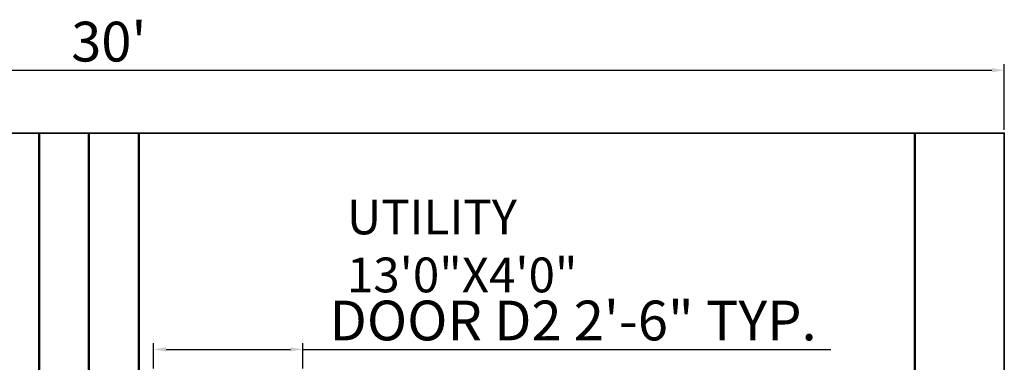
# Model space of a CAD drawing. Units: inches. Extents: x 1986 to 21484, y -1816 to 2016.
# Tile 79 of 85: x 3701 to 3899, y 1855 to 1924. Entities that reach past the tile are written whole.
import ezdxf

# ---------------------------------------------------------------- set-up
doc = ezdxf.new("R2010")
doc.units = ezdxf.units.IN
for name, color, linetype, lineweight in [('A-ANNO-DIMS', 2, 'Continuous', 18), ('A-AREA-IDEN', 3, 'Continuous', 18), ('A-WALL', 7, 'Continuous', 50), ('A-WALL-PATT', 8, 'Continuous', 13), ('C-PROP', 7, 'Continuous', 35)]:
    doc.layers.add(name, color=color, linetype=linetype, lineweight=lineweight)
doc.styles.get("Standard").update_dxf_attribs({"font": 'arial.ttf'})
doc.dimstyles.new('ISO-25', dxfattribs={"dimtxt": 8, "dimasz": 2.5, "dimexe": 1.25, "dimexo": 0.625, "dimtad": 1, "dimdec": 1, "dimlunit": 3, "dimtxsty": 'Standard', "dimcen": 2.5, "dimadec": 0, "dimazin": 0, "dimtfac": 1, "dimtdec": 1, "dimtmove": 0, "dimatfit": 3, "dimfxl": 1, "dimarcsym": 0})

# ---------------------------------------------------------------- blocks, each defined once
blk = doc.blocks.new('*D33')
at = {"layer": 'A-ANNO-DIMS', "color": 0, "lineweight": -2, "transparency": 16777216}
for p, q in [((3538.91, 1901.38), (3538.91, 1914.65)), ((3898.91, 1901.38), (3898.91, 1914.65)), ((3541.41, 1913.4), (3896.41, 1913.4))]:
    blk.add_line(p, q, dxfattribs=at)
at = {"layer": 'A-ANNO-DIMS', "color": 0, "transparency": 16777216}
for points in [[(3541.41, 1913.82), (3541.41, 1912.99), (3538.91, 1913.4)], [(3896.41, 1913.82), (3896.41, 1912.99), (3898.91, 1913.4)]]:
    blk.add_solid(points, dxfattribs=at)
at = {"layer": 'Defpoints', "color": 0, "transparency": 16777216}
for p in [(3898.91, 1913.4), (3538.91, 1900.75), (3898.91, 1900.75)]:
    blk.add_point(p, dxfattribs=at)
at = {"layer": 'A-ANNO-DIMS', "color": 0, "transparency": 16777216, "insert": (3718.91, 1918.12), "char_height": 8, "attachment_point": 5}
blk.add_mtext("30'", dxfattribs=at)
blk = doc.blocks.new('*D91')
at = {"layer": 'A-ANNO-DIMS', "color": 0, "lineweight": -2, "transparency": 16777216}
for p, q in [((3727.91, 1853.38), (3727.91, 1858.5)), ((3757.91, 1853.38), (3757.91, 1858.5)), ((3730.41, 1857.25), (3755.41, 1857.25)), ((3757.91, 1857.25), (3864.05, 1857.25))]:
    blk.add_line(p, q, dxfattribs=at)
at = {"layer": 'A-ANNO-DIMS', "color": 0, "transparency": 16777216}
for points in [[(3730.41, 1857.67), (3730.41, 1856.84), (3727.91, 1857.25)], [(3755.41, 1857.67), (3755.41, 1856.84), (3757.91, 1857.25)]]:
    blk.add_solid(points, dxfattribs=at)
at = {"layer": 'Defpoints', "color": 0, "transparency": 16777216}
for p in [(3757.91, 1857.25), (3727.91, 1852.75), (3757.91, 1852.75)]:
    blk.add_point(p, dxfattribs=at)
at = {"layer": 'A-ANNO-DIMS', "color": 0, "transparency": 16777216, "insert": (3812.23, 1862.02), "char_height": 8, "attachment_point": 5}
blk.add_mtext('DOOR D2 2\'-6" TYP.', dxfattribs=at)

msp = doc.modelspace()

# ---------------------------------------------------------------- hatches: boundary and pattern name
at = {"layer": 'A-WALL-PATT'}
h = msp.add_hatch(dxfattribs=at)
h.set_pattern_fill('ANSI32', color=256, scale=0.5)
h.paths.add_polyline_path([(3631.91, 1852.75), (3574.91, 1852.75), (3574.91, 1753.75), (3583.91, 1753.75), (3583.91, 1843.75), (3631.91, 1843.75)])
h.paths.add_polyline_path([(3727.91, 1852.75), (3673.91, 1852.75), (3673.91, 1843.75), (3721.91, 1843.75), (3721.91, 1627.75), (3727.91, 1627.75)])
h.paths.add_polyline_path([(3880.91, 1852.75), (3757.91, 1852.75), (3757.91, 1843.75), (3871.91, 1843.75), (3871.91, 1795.75), (3775.91, 1795.75), (3775.91, 1813.75), (3769.91, 1813.75), (3769.91, 1789.75), (3871.91, 1789.75), (3871.91, 1741.75), (3880.91, 1741.75)])
h.paths.add_polyline_path([(3880.91, 1705.75), (3871.91, 1705.75), (3871.91, 1600.75), (3880.91, 1600.75)])
h.paths.add_polyline_path([(3685.91, 1687.75), (3583.91, 1687.75), (3583.91, 1711.75), (3574.91, 1711.75), (3574.91, 1669.75), (3583.91, 1669.75), (3583.91, 1681.75), (3673.91, 1681.75), (3673.91, 1663.75), (3679.91, 1663.75), (3679.91, 1681.75), (3685.91, 1681.75)])
h.paths.add_polyline_path([(3583.91, 1399.75), (3574.91, 1399.75), (3574.91, 1276.75), (3583.91, 1276.75)])
h.paths.add_polyline_path([(3648.41, 1387.75), (3631.91, 1387.75), (3631.91, 1378.75), (3648.41, 1378.75)])
h.paths.add_polyline_path([(3715.91, 1387.75), (3690.41, 1387.75), (3690.41, 1378.75), (3706.91, 1378.75), (3706.91, 1189.75), (3715.91, 1189.75)])
h.paths.add_polyline_path([(3880.91, 1387.75), (3871.91, 1387.75), (3751.91, 1387.75), (3751.91, 1381.75), (3871.91, 1381.75), (3871.91, 1363.75), (3880.91, 1363.75)])
h.paths.add_polyline_path([(3880.91, 1441.75), (3871.91, 1441.75), (3871.91, 1423.75), (3880.91, 1423.75)])
h.paths.add_polyline_path([(3880.91, 1495.75), (3871.91, 1495.75), (3871.91, 1477.75), (3880.91, 1477.75)])
h.paths.add_polyline_path([(3880.91, 1339.75), (3871.91, 1339.75), (3871.91, 1321.75), (3775.91, 1321.75), (3775.91, 1351.75), (3769.91, 1351.75), (3769.91, 1315.75), (3871.91, 1315.75), (3871.91, 1303.75), (3880.91, 1303.75)])
h.paths.add_polyline_path([(3880.91, 1261.75), (3871.91, 1261.75), (3871.91, 1189.75), (3880.91, 1189.75)])
h.paths.add_polyline_path([(3880.91, 1147.75), (3871.91, 1147.75), (3871.91, 1123.75), (3763.91, 1123.75), (3763.91, 1114.75), (3880.91, 1114.75)])
h.paths.add_polyline_path([(3721.91, 1123.75), (3715.91, 1123.75), (3715.91, 1147.75), (3706.91, 1147.75), (3706.91, 1114.75), (3721.91, 1114.75)])
h.paths.add_polyline_path([(3880.91, 1564.75), (3871.91, 1564.75), (3871.91, 1537.75), (3789.91, 1537.75), (3789.91, 1531.75), (3871.91, 1531.75), (3880.91, 1531.75)])
h.paths.add_polyline_path([(3583.91, 1627.75), (3679.91, 1627.75), (3679.91, 1633.75), (3649.91, 1633.75), (3583.91, 1633.75), (3583.91, 1645.75), (3574.91, 1645.75), (3574.91, 1441.75), (3583.91, 1441.75)])
h.paths.add_polyline_path([(3733.26, 1736.83), (3733.26, 1685.78), (3741.8, 1685.78), (3741.8, 1736.83)], flags=9)
h.paths.add_polyline_path([(3763.81, 1864.73), (3812.77, 1864.73), (3812.77, 1891.35), (3763.81, 1891.35)], flags=9)
h.paths.add_polyline_path([(3797.97, 1806.84), (3841.79, 1806.84), (3841.79, 1833.45), (3797.97, 1833.45)], flags=25)
h.paths.add_polyline_path([(3779.25, 1690.08), (3833.38, 1690.08), (3833.38, 1716.69), (3779.25, 1716.69)], flags=9)
h.paths.add_polyline_path([(3805.23, 1565.41), (3849.03, 1565.41), (3849.03, 1592.03), (3805.23, 1592.03)], flags=9)
h.paths.add_polyline_path([(3638.57, 1496.24), (3711.25, 1496.24), (3711.25, 1522.85), (3638.57, 1522.85)], flags=9)
h.paths.add_polyline_path([(3617.97, 1320.51), (3666.93, 1320.51), (3666.93, 1347.12), (3617.97, 1347.12)], flags=9)
h.paths.add_polyline_path([(3768.51, 1208.98), (3836.51, 1208.98), (3836.51, 1235.59), (3768.51, 1235.59)], flags=9)
h.paths.add_polyline_path([(3791.7, 1338.54), (3844.53, 1338.54), (3844.53, 1365.15), (3791.7, 1365.15)], flags=9)
h.paths.add_polyline_path([(3614.85, 1758.76), (3671.08, 1758.76), (3671.08, 1785.38), (3614.85, 1785.38)], flags=9)
h.paths.add_polyline_path([(3603.38, 1642.68), (3655.11, 1642.68), (3655.11, 1669.29), (3603.38, 1669.29)], flags=9)

# ---------------------------------------------------------------- linework, layer by layer
at = {"layer": 'A-WALL'}
for p, q in [((3704.91, 1900.75), (3704.91, 1852.75)), ((3714.91, 1900.75), (3714.91, 1852.75)), ((3724.91, 1900.75), (3724.91, 1852.75)), ((3880.91, 1900.75), (3880.91, 1114.75))]:
    msp.add_line(p, q, dxfattribs=at)
at = {"layer": 'C-PROP'}
msp.add_lwpolyline([(3538.91, 1900.75), (3898.91, 1900.75), (3898.91, 1066.75), (3538.91, 1066.75)], close=True, dxfattribs=at)

# ---------------------------------------------------------------- texts
at = {"layer": 'A-AREA-IDEN', "insert": (3766.77, 1887.39), "char_height": 7, "attachment_point": 1}
msp.add_mtext_dynamic_manual_height_columns('{\\fTimes New Roman|b0|i0|c0|p18;UTILITY\\P13\'0"X4\'0"}', width=105.6127, gutter_width=12.5, heights=[0], dxfattribs=at)

# ---------------------------------------------------------------- dimensions: what is measured, and where the dimension line sits
at = {"layer": 'A-ANNO-DIMS'}
dim = msp.add_linear_dim(base=(3898.91, 1913.4), p1=(3538.91, 1900.75), p2=(3898.91, 1900.75), dimstyle='ISO-25', override={"dimclrd": 0, "dimclre": 0, "dimclrt": 0}, dxfattribs=at)
dim.commit()
dim.dimension.update_dxf_attribs({"geometry": '*D33', "text_midpoint": (3718.91, 1918.12)})
dim = msp.add_linear_dim(base=(3757.91, 1857.25), p1=(3727.91, 1852.75), p2=(3757.91, 1852.75), text='DOOR D2 <> TYP.', dimstyle='ISO-25', override={"dimdec": 1, "dimrnd": 0, "dimzin": 1, "dimlunit": 4, "dimfrac": 2}, dxfattribs=at)
dim.commit()
dim.dimension.update_dxf_attribs({"geometry": '*D91', "text_midpoint": (3812.23, 1862.02)})

doc.saveas('drawing.dxf')
